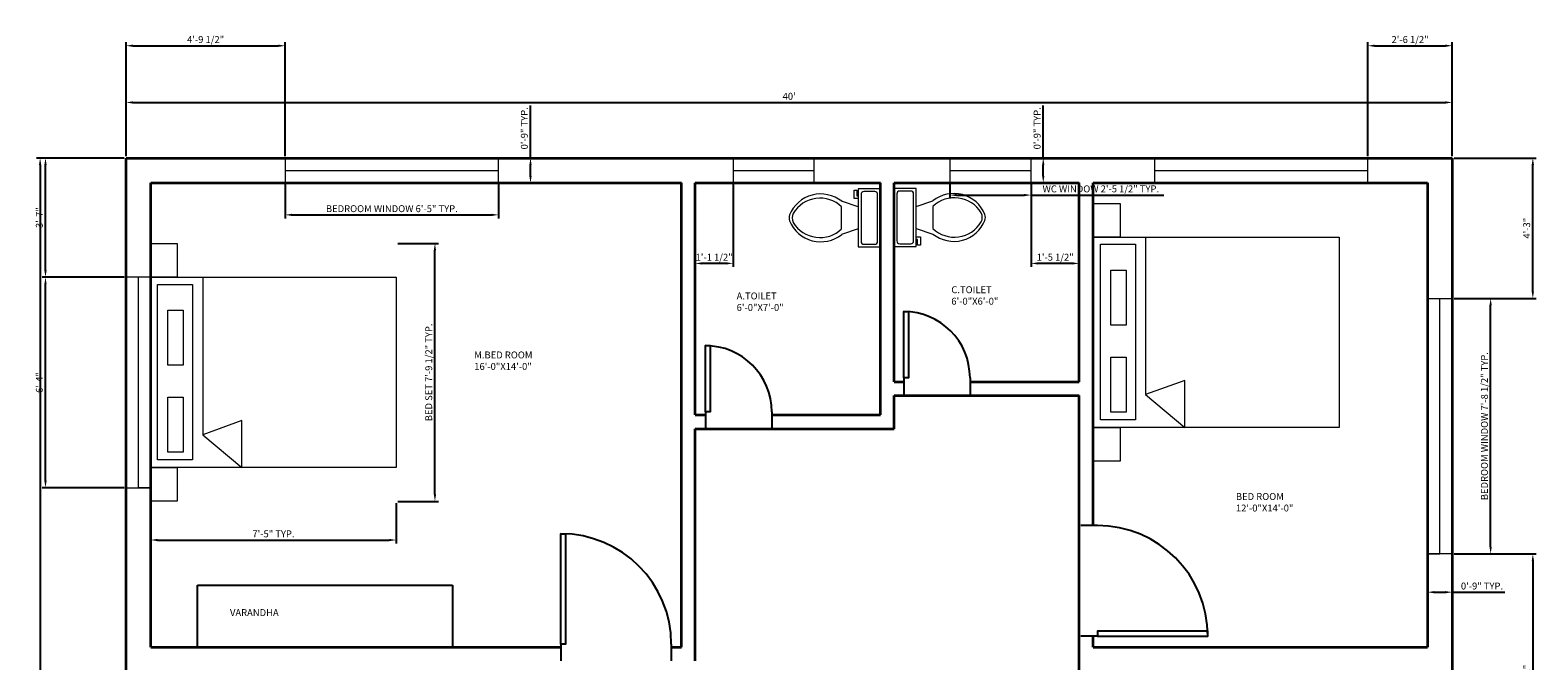
# Model space of a CAD drawing. Units: inches. Extents: x 2981 to 3526, y 1512 to 2158.
# Tile 4 of 4: x 2981 to 3526, y 1930 to 2158. Entities that reach past the tile are written whole.
import ezdxf

# ---------------------------------------------------------------- set-up
doc = ezdxf.new("R2010")
doc.units = ezdxf.units.IN
for name, color, linetype, lineweight in [('A-ANNO-DIMS', 2, 'Continuous', 18), ('A-AREA-IDEN', 7, 'Continuous', 18), ('A-DOOR', 4, 'Continuous', 25), ('A-FLOR', 7, 'Continuous', 25), ('A-FLOR-FIXT', 9, 'Continuous', 18), ('A-FURN', 8, 'Continuous', 18), ('A-GLAZ', 4, 'Continuous', 18), ('A-WALL', 7, 'Continuous', 35)]:
    doc.layers.add(name, color=color, linetype=linetype, lineweight=lineweight)
doc.styles.get("Standard").update_dxf_attribs({"font": 'arial.ttf'})
doc.dimstyles.new('ISO-25', dxfattribs={"dimtxt": 2.5, "dimasz": 2.5, "dimexe": 1.25, "dimexo": 0.625, "dimtad": 1, "dimlunit": 3, "dimtxsty": 'Standard', "dimcen": 2.5, "dimadec": 0, "dimazin": 0, "dimtfac": 1, "dimtmove": 0, "dimatfit": 3, "dimfxl": 1, "dimarcsym": 0})

# ---------------------------------------------------------------- blocks, each defined once
blk = doc.blocks.new('*U2')
for p, q in [((0, 0), (0, -6)), ((40, 0), (40, -6))]:
    blk.add_line(p, q)
blk.add_lwpolyline([(0, 0), (0, 40), (1.75, 40), (1.75, 0)], close=True)
blk.add_arc((0, 0), 40, 0, 90)
blk = doc.blocks.new('*U3')
for p, q in [((0, 0), (0, -6)), ((-40, 0), (-40, -6))]:
    blk.add_line(p, q)
blk.add_lwpolyline([(0, 0), (0, 40), (-1.75, 40), (-1.75, 0)], close=True)
blk.add_arc((0, 0), 40, 90, 180)
blk = doc.blocks.new('*U5')
for p, q in [((0, 0), (0, -6)), ((24, 0), (24, -6))]:
    blk.add_line(p, q)
blk.add_lwpolyline([(0, 0), (0, 24), (1.75, 24), (1.75, 0)], close=True)
blk.add_arc((0, 0), 24, 0, 90)
blk = doc.blocks.new('*U9')
for p, q in [((9.5, -6), (9.5, -2)), ((-10, -8.5), (-8, -8.5)), ((-10, -9.5), (-10, -8.5)), ((-7, -9.5), (-10, -9.5)), ((-8, -8.5), (-8, -8)), ((-7, -8), (-7, -9.5)), ((-4, -8), (-6, -14)), ((4, -8), (6, -14)), ((4, -14), (-4, -14))]:
    blk.add_line(p, q)
blk.add_lwpolyline([(10.5, -8), (10.5, 0), (-10.5, 0), (-10.5, -8)], close=True)
for points in [[(-9.5, -2), (-9.5, -6)], [(8.5, -1), (-8.5, -1)], [(-8.5, -7), (8.5, -7)]]:
    blk.add_lwpolyline(points)
for centre, radius, start, end in [((-8.62, -1.88), 0.884, 81.8699, 188.1301), ((8.62, -1.88), 0.884, 351.8699, 98.1301), ((-8.62, -6.12), 0.884, 171.8699, 278.1301), ((8.62, -6.12), 0.884, 261.8699, 8.1301), ((3.52, -21.58), 12.17, 141.4691, 247.9714), ((4.2, -21.82), 11.33, 136.3677, 238.9468), ((-3.52, -21.58), 12.17, 292.0284, 38.5307), ((-4.2, -21.82), 11.33, 301.053, 43.6321), ((0, -27.88), 4, 245.7318, 294.2682), ((0, -29), 4, 254.8605, 285.1395)]:
    blk.add_arc(centre, radius, start, end)
blk = doc.blocks.new('*D14')
at = {"layer": 'A-ANNO-DIMS', "color": 0, "lineweight": -2, "transparency": 16777216}
for p, q in [((3015.4, 2112.83), (3015.4, 2133.57)), ((3495.4, 2112.83), (3495.4, 2133.57)), ((3017.9, 2132.32), (3492.9, 2132.32))]:
    blk.add_line(p, q, dxfattribs=at)
at = {"layer": 'A-ANNO-DIMS', "color": 0, "transparency": 16777216}
for points in [[(3017.9, 2132.73), (3017.9, 2131.9), (3015.4, 2132.32)], [(3492.9, 2132.73), (3492.9, 2131.9), (3495.4, 2132.32)]]:
    blk.add_solid(points, dxfattribs=at)
at = {"layer": 'Defpoints', "color": 0, "transparency": 16777216}
for p in [(3495.4, 2132.32), (3015.4, 2112.2), (3495.4, 2112.2)]:
    blk.add_point(p, dxfattribs=at)
at = {"layer": 'A-ANNO-DIMS', "color": 0, "transparency": 16777216, "insert": (3255.4, 2134.22), "char_height": 2.5, "attachment_point": 5}
blk.add_mtext("40'", dxfattribs=at)
blk = doc.blocks.new('*D15')
at = {"layer": 'A-ANNO-DIMS', "color": 0, "lineweight": -2, "transparency": 16777216}
for p, q in [((3014.77, 2112.2), (2983.05, 2112.2)), ((2984.3, 2109.7), (2984.3, 1574.7)), ((3014.77, 1572.2), (2983.05, 1572.2))]:
    blk.add_line(p, q, dxfattribs=at)
at = {"layer": 'A-ANNO-DIMS', "color": 0, "transparency": 16777216}
for points in [[(2983.89, 2109.7), (2984.72, 2109.7), (2984.3, 2112.2)], [(2983.89, 1574.7), (2984.72, 1574.7), (2984.3, 1572.2)]]:
    blk.add_solid(points, dxfattribs=at)
at = {"layer": 'Defpoints', "color": 0, "transparency": 16777216}
for p in [(3015.4, 2112.2), (2984.3, 1572.2), (3015.4, 1572.2)]:
    blk.add_point(p, dxfattribs=at)
at = {"layer": 'A-ANNO-DIMS', "color": 0, "transparency": 16777216, "insert": (2982.41, 1842.2), "char_height": 2.5, "attachment_point": 5, "rotation": 90}
blk.add_mtext("45'", dxfattribs=at)
blk = doc.blocks.new('WIN-77IN-BEDROOM')
for p, q in [((0, 9), (0, 0)), ((77.2, 9), (0, 9)), ((0, 9), (0, 4.5)), ((77.2, 0), (77.2, 9)), ((0, 4.5), (77.2, 4.5)), ((0, 0), (77.2, 0))]:
    blk.add_line(p, q)
blk = doc.blocks.new('WIN-29IN-TOILET')
for p, q in [((0, 9), (0, 0)), ((29.42, 9), (0, 9)), ((0, 9), (0, 4.5)), ((29.42, 0), (29.42, 9)), ((0, 4.5), (29.42, 4.5)), ((0, 0), (29.42, 0))]:
    blk.add_line(p, q)
blk = doc.blocks.new('WIN-92IN-BEDROOM')
for p, q in [((0, 92.47), (9, 92.47)), ((0, 92.47), (0, 0)), ((4.5, 0), (4.5, 92.47)), ((9, 92.47), (9, 0)), ((9, 0), (0, 0)), ((0, 0), (4.5, 0))]:
    blk.add_line(p, q)
blk = doc.blocks.new('BED-DOUBLE-WITH-NIGHTSTANDS')
for p, q in [((18.84, 81.09), (18.84, 24.12)), ((33.02, 29.21), (18.84, 24.12)), ((33.02, 12.24), (33.02, 29.21)), ((18.84, 24.12), (33.02, 12.24))]:
    blk.add_line(p, q)
for points in [[(9.63, 93.35), (9.63, 81.1), (0.08, 81.1), (0.08, 93.35)], [(0.08, 12.24), (0.08, 81.09), (88.86, 81.09), (88.86, 12.24)], [(2.5, 15.01), (2.5, 78.54), (15.13, 78.54), (15.13, 15.01)], [(6.2, 49.25), (6.2, 69.14), (11.74, 69.14), (11.74, 49.25)], [(6.2, 17.79), (6.2, 37.68), (11.74, 37.68), (11.74, 17.79)], [(9.63, 12.24), (9.63, 0), (0, 0), (0, 12.24)]]:
    blk.add_lwpolyline(points, close=True)
blk = doc.blocks.new('*D21')
at = {"layer": 'A-ANNO-DIMS', "color": 0, "lineweight": -2, "transparency": 16777216}
for p, q in [((3113.82, 2081.29), (3128.45, 2081.29)), ((3127.2, 1990.44), (3127.2, 2078.79)), ((3113.82, 1987.94), (3128.45, 1987.94))]:
    blk.add_line(p, q, dxfattribs=at)
at = {"layer": 'A-ANNO-DIMS', "color": 0, "transparency": 16777216}
for points in [[(3126.78, 2078.79), (3127.61, 2078.79), (3127.2, 2081.29)], [(3126.78, 1990.44), (3127.61, 1990.44), (3127.2, 1987.94)]]:
    blk.add_solid(points, dxfattribs=at)
at = {"layer": 'Defpoints', "color": 0, "transparency": 16777216}
for p in [(3113.19, 2081.29), (3127.2, 2081.29), (3113.19, 1987.94)]:
    blk.add_point(p, dxfattribs=at)
at = {"layer": 'A-ANNO-DIMS', "color": 0, "transparency": 16777216, "insert": (3125.28, 2034.62), "char_height": 2.5, "attachment_point": 5, "rotation": 90}
blk.add_mtext('BED SET 7\'-9 1/2" TYP.', dxfattribs=at)
blk = doc.blocks.new('*D22')
at = {"layer": 'A-ANNO-DIMS', "color": 0, "lineweight": -2, "transparency": 16777216}
for p, q in [((3024.33, 1987.32), (3024.33, 1972.69)), ((3113.19, 1987.32), (3113.19, 1972.69)), ((3026.83, 1973.94), (3110.69, 1973.94))]:
    blk.add_line(p, q, dxfattribs=at)
at = {"layer": 'A-ANNO-DIMS', "color": 0, "transparency": 16777216}
for points in [[(3026.83, 1974.36), (3026.83, 1973.53), (3024.33, 1973.94)], [(3110.69, 1974.36), (3110.69, 1973.53), (3113.19, 1973.94)]]:
    blk.add_solid(points, dxfattribs=at)
at = {"layer": 'Defpoints', "color": 0, "transparency": 16777216}
for p in [(3024.33, 1987.94), (3113.19, 1987.94), (3113.19, 1973.94)]:
    blk.add_point(p, dxfattribs=at)
at = {"layer": 'A-ANNO-DIMS', "color": 0, "transparency": 16777216, "insert": (3068.76, 1975.84), "char_height": 2.5, "attachment_point": 5}
blk.add_mtext('7\'-5" TYP.', dxfattribs=at)
blk = doc.blocks.new('*D27')
at = {"layer": 'A-ANNO-DIMS', "color": 0, "lineweight": -2, "transparency": 16777216}
for p, q in [((3073, 2102.58), (3073, 2090.37)), ((3150.2, 2102.58), (3150.2, 2090.37)), ((3075.5, 2091.62), (3147.7, 2091.62))]:
    blk.add_line(p, q, dxfattribs=at)
at = {"layer": 'A-ANNO-DIMS', "color": 0, "transparency": 16777216}
for points in [[(3075.5, 2092.04), (3075.5, 2091.21), (3073, 2091.62)], [(3147.7, 2092.04), (3147.7, 2091.21), (3150.2, 2091.62)]]:
    blk.add_solid(points, dxfattribs=at)
at = {"layer": 'Defpoints', "color": 0, "transparency": 16777216}
for p in [(3073, 2103.2), (3150.2, 2103.2), (3150.2, 2091.62)]:
    blk.add_point(p, dxfattribs=at)
at = {"layer": 'A-ANNO-DIMS', "color": 0, "transparency": 16777216, "insert": (3111.6, 2093.54), "char_height": 2.5, "attachment_point": 5}
blk.add_mtext('BEDROOM WINDOW 6\'-5" TYP.', dxfattribs=at)
blk = doc.blocks.new('*D28')
at = {"layer": 'A-ANNO-DIMS', "color": 0, "lineweight": -2, "transparency": 16777216}
for p, q in [((3161.78, 2112.2), (3161.78, 2131.19)), ((3150.83, 2112.2), (3163.03, 2112.2)), ((3161.78, 2105.7), (3161.78, 2109.7)), ((3150.83, 2103.2), (3163.03, 2103.2))]:
    blk.add_line(p, q, dxfattribs=at)
at = {"layer": 'A-ANNO-DIMS', "color": 0, "transparency": 16777216}
for points in [[(3161.37, 2109.7), (3162.2, 2109.7), (3161.78, 2112.2)], [(3161.37, 2105.7), (3162.2, 2105.7), (3161.78, 2103.2)]]:
    blk.add_solid(points, dxfattribs=at)
at = {"layer": 'Defpoints', "color": 0, "transparency": 16777216}
for p in [(3150.2, 2112.2), (3161.78, 2112.2), (3150.2, 2103.2)]:
    blk.add_point(p, dxfattribs=at)
at = {"layer": 'A-ANNO-DIMS', "color": 0, "transparency": 16777216, "insert": (3159.88, 2122.95), "char_height": 2.5, "attachment_point": 5, "rotation": 90}
blk.add_mtext('0\'-9" TYP.', dxfattribs=at)
blk = doc.blocks.new('*D29')
at = {"layer": 'A-ANNO-DIMS', "color": 0, "lineweight": -2, "transparency": 16777216}
for p, q in [((3313.51, 2102.58), (3313.51, 2097.54)), ((3342.94, 2102.58), (3342.94, 2097.54)), ((3316.01, 2098.79), (3340.44, 2098.79)), ((3342.94, 2098.79), (3390.94, 2098.79))]:
    blk.add_line(p, q, dxfattribs=at)
at = {"layer": 'A-ANNO-DIMS', "color": 0, "transparency": 16777216}
for points in [[(3316.01, 2099.21), (3316.01, 2098.37), (3313.51, 2098.79)], [(3340.44, 2099.21), (3340.44, 2098.37), (3342.94, 2098.79)]]:
    blk.add_solid(points, dxfattribs=at)
at = {"layer": 'Defpoints', "color": 0, "transparency": 16777216}
for p in [(3313.51, 2103.2), (3342.94, 2103.2), (3342.94, 2098.79)]:
    blk.add_point(p, dxfattribs=at)
at = {"layer": 'A-ANNO-DIMS', "color": 0, "transparency": 16777216, "insert": (3368.19, 2100.71), "char_height": 2.5, "attachment_point": 5}
blk.add_mtext('WC WINDOW 2\'-5 1/2" TYP.', dxfattribs=at)
blk = doc.blocks.new('*D30')
at = {"layer": 'A-ANNO-DIMS', "color": 0, "lineweight": -2, "transparency": 16777216}
for p, q in [((3347.35, 2112.2), (3347.35, 2131.19)), ((3343.57, 2112.2), (3348.6, 2112.2)), ((3347.35, 2105.7), (3347.35, 2109.7)), ((3343.57, 2103.2), (3348.6, 2103.2))]:
    blk.add_line(p, q, dxfattribs=at)
at = {"layer": 'A-ANNO-DIMS', "color": 0, "transparency": 16777216}
for points in [[(3346.94, 2109.7), (3347.77, 2109.7), (3347.35, 2112.2)], [(3346.94, 2105.7), (3347.77, 2105.7), (3347.35, 2103.2)]]:
    blk.add_solid(points, dxfattribs=at)
at = {"layer": 'Defpoints', "color": 0, "transparency": 16777216}
for p in [(3342.94, 2112.2), (3347.35, 2112.2), (3342.94, 2103.2)]:
    blk.add_point(p, dxfattribs=at)
at = {"layer": 'A-ANNO-DIMS', "color": 0, "transparency": 16777216, "insert": (3345.45, 2122.95), "char_height": 2.5, "attachment_point": 5, "rotation": 90}
blk.add_mtext('0\'-9" TYP.', dxfattribs=at)
blk = doc.blocks.new('*D31')
at = {"layer": 'A-ANNO-DIMS', "color": 0, "lineweight": -2, "transparency": 16777216}
for p, q in [((3496.02, 2061.39), (3510.52, 2061.39)), ((3509.27, 1971.43), (3509.27, 2058.89)), ((3496.02, 1968.93), (3510.52, 1968.93))]:
    blk.add_line(p, q, dxfattribs=at)
at = {"layer": 'A-ANNO-DIMS', "color": 0, "transparency": 16777216}
for points in [[(3508.85, 2058.89), (3509.69, 2058.89), (3509.27, 2061.39)], [(3508.85, 1971.43), (3509.69, 1971.43), (3509.27, 1968.93)]]:
    blk.add_solid(points, dxfattribs=at)
at = {"layer": 'Defpoints', "color": 0, "transparency": 16777216}
for p in [(3495.4, 2061.39), (3509.27, 2061.39), (3495.4, 1968.93)]:
    blk.add_point(p, dxfattribs=at)
at = {"layer": 'A-ANNO-DIMS', "color": 0, "transparency": 16777216, "insert": (3507.35, 2015.16), "char_height": 2.5, "attachment_point": 5, "rotation": 90}
blk.add_mtext('BEDROOM WINDOW 7\'-8 1/2" TYP.', dxfattribs=at)
blk = doc.blocks.new('*D32')
at = {"layer": 'A-ANNO-DIMS', "color": 0, "lineweight": -2, "transparency": 16777216}
for p, q in [((3486.4, 1968.3), (3486.4, 1953.81)), ((3495.4, 1968.3), (3495.4, 1953.81)), ((3488.9, 1955.06), (3492.9, 1955.06)), ((3495.4, 1955.06), (3514.39, 1955.06))]:
    blk.add_line(p, q, dxfattribs=at)
at = {"layer": 'A-ANNO-DIMS', "color": 0, "transparency": 16777216}
for points in [[(3488.9, 1955.47), (3488.9, 1954.64), (3486.4, 1955.06)], [(3492.9, 1955.47), (3492.9, 1954.64), (3495.4, 1955.06)]]:
    blk.add_solid(points, dxfattribs=at)
at = {"layer": 'Defpoints', "color": 0, "transparency": 16777216}
for p in [(3486.4, 1968.93), (3495.4, 1968.93), (3495.4, 1955.06)]:
    blk.add_point(p, dxfattribs=at)
at = {"layer": 'A-ANNO-DIMS', "color": 0, "transparency": 16777216, "insert": (3506.14, 1956.96), "char_height": 2.5, "attachment_point": 5}
blk.add_mtext('0\'-9" TYP.', dxfattribs=at)
blk = doc.blocks.new('*D41')
at = {"layer": 'A-ANNO-DIMS', "color": 0, "lineweight": -2, "transparency": 16777216}
for p, q in [((3496.02, 2112.2), (3525.79, 2112.2)), ((3524.54, 2063.89), (3524.54, 2109.7)), ((3496.02, 2061.39), (3525.79, 2061.39))]:
    blk.add_line(p, q, dxfattribs=at)
at = {"layer": 'A-ANNO-DIMS', "color": 0, "transparency": 16777216}
for points in [[(3524.13, 2109.7), (3524.96, 2109.7), (3524.54, 2112.2)], [(3524.13, 2063.89), (3524.96, 2063.89), (3524.54, 2061.39)]]:
    blk.add_solid(points, dxfattribs=at)
at = {"layer": 'Defpoints', "color": 0, "transparency": 16777216}
for p in [(3495.4, 2112.2), (3524.54, 2112.2), (3495.4, 2061.39)]:
    blk.add_point(p, dxfattribs=at)
at = {"layer": 'A-ANNO-DIMS', "color": 0, "transparency": 16777216, "insert": (3522.64, 2086.8), "char_height": 2.5, "attachment_point": 5, "rotation": 90}
blk.add_mtext('4\'-3"', dxfattribs=at)
blk = doc.blocks.new('*D42')
at = {"layer": 'A-ANNO-DIMS', "color": 0, "lineweight": -2, "transparency": 16777216}
for p, q in [((3496.02, 1968.93), (3525.79, 1968.93)), ((3524.54, 1966.43), (3524.54, 1875.83)), ((3496.02, 1873.33), (3525.79, 1873.33))]:
    blk.add_line(p, q, dxfattribs=at)
at = {"layer": 'A-ANNO-DIMS', "color": 0, "transparency": 16777216}
for points in [[(3524.13, 1966.43), (3524.96, 1966.43), (3524.54, 1968.93)], [(3524.13, 1875.83), (3524.96, 1875.83), (3524.54, 1873.33)]]:
    blk.add_solid(points, dxfattribs=at)
at = {"layer": 'Defpoints', "color": 0, "transparency": 16777216}
for p in [(3495.4, 1968.93), (3495.4, 1873.33), (3524.54, 1873.33)]:
    blk.add_point(p, dxfattribs=at)
at = {"layer": 'A-ANNO-DIMS', "color": 0, "transparency": 16777216, "insert": (3522.63, 1921.13), "char_height": 2.5, "attachment_point": 5, "rotation": 90}
blk.add_mtext('7\'-11 1/2"', dxfattribs=at)
blk = doc.blocks.new('*D43')
at = {"layer": 'A-ANNO-DIMS', "color": 0, "lineweight": -2, "transparency": 16777216}
for p, q in [((3014.77, 2069.05), (2985, 2069.05)), ((2986.25, 1995.38), (2986.25, 2066.55)), ((3014.77, 1992.88), (2985, 1992.88))]:
    blk.add_line(p, q, dxfattribs=at)
at = {"layer": 'A-ANNO-DIMS', "color": 0, "transparency": 16777216}
for points in [[(2985.84, 2066.55), (2986.67, 2066.55), (2986.25, 2069.05)], [(2985.84, 1995.38), (2986.67, 1995.38), (2986.25, 1992.88)]]:
    blk.add_solid(points, dxfattribs=at)
at = {"layer": 'Defpoints', "color": 0, "transparency": 16777216}
for p in [(2986.25, 2069.05), (3015.4, 2069.05), (3015.4, 1992.88)]:
    blk.add_point(p, dxfattribs=at)
at = {"layer": 'A-ANNO-DIMS', "color": 0, "transparency": 16777216, "insert": (2984.35, 2030.96), "char_height": 2.5, "attachment_point": 5, "rotation": 90}
blk.add_mtext('6\'-4"', dxfattribs=at)
blk = doc.blocks.new('*D46')
at = {"layer": 'A-ANNO-DIMS', "color": 0, "lineweight": -2, "transparency": 16777216}
for p, q in [((3015.4, 2112.83), (3015.4, 2154.09)), ((3017.9, 2152.84), (3070.5, 2152.84)), ((3073, 2112.83), (3073, 2154.09))]:
    blk.add_line(p, q, dxfattribs=at)
at = {"layer": 'A-ANNO-DIMS', "color": 0, "transparency": 16777216}
for points in [[(3017.9, 2153.26), (3017.9, 2152.42), (3015.4, 2152.84)], [(3070.5, 2153.26), (3070.5, 2152.42), (3073, 2152.84)]]:
    blk.add_solid(points, dxfattribs=at)
at = {"layer": 'Defpoints', "color": 0, "transparency": 16777216}
for p in [(3073, 2152.84), (3015.4, 2112.2), (3073, 2112.2)]:
    blk.add_point(p, dxfattribs=at)
at = {"layer": 'A-ANNO-DIMS', "color": 0, "transparency": 16777216, "insert": (3044.2, 2154.76), "char_height": 2.5, "attachment_point": 5}
blk.add_mtext('4\'-9 1/2"', dxfattribs=at)
blk = doc.blocks.new('*D47')
at = {"layer": 'A-ANNO-DIMS', "color": 0, "lineweight": -2, "transparency": 16777216}
for p, q in [((3221.4, 2102.58), (3221.4, 2072.81)), ((3235.08, 2102.58), (3235.08, 2072.81)), ((3232.58, 2074.06), (3223.9, 2074.06))]:
    blk.add_line(p, q, dxfattribs=at)
at = {"layer": 'A-ANNO-DIMS', "color": 0, "transparency": 16777216}
for points in [[(3223.9, 2074.47), (3223.9, 2073.64), (3221.4, 2074.06)], [(3232.58, 2074.47), (3232.58, 2073.64), (3235.08, 2074.06)]]:
    blk.add_solid(points, dxfattribs=at)
at = {"layer": 'Defpoints', "color": 0, "transparency": 16777216}
for p in [(3221.4, 2103.2), (3235.08, 2103.2), (3221.4, 2074.06)]:
    blk.add_point(p, dxfattribs=at)
at = {"layer": 'A-ANNO-DIMS', "color": 0, "transparency": 16777216, "insert": (3228.24, 2075.98), "char_height": 2.5, "attachment_point": 5}
blk.add_mtext('1\'-1 1/2"', dxfattribs=at)
blk = doc.blocks.new('*D48')
at = {"layer": 'A-ANNO-DIMS', "color": 0, "lineweight": -2, "transparency": 16777216}
for p, q in [((3342.94, 2102.58), (3342.94, 2072.81)), ((3360.4, 2102.58), (3360.4, 2072.81)), ((3357.9, 2074.06), (3345.44, 2074.06))]:
    blk.add_line(p, q, dxfattribs=at)
at = {"layer": 'A-ANNO-DIMS', "color": 0, "transparency": 16777216}
for points in [[(3345.44, 2074.47), (3345.44, 2073.64), (3342.94, 2074.06)], [(3357.9, 2074.47), (3357.9, 2073.64), (3360.4, 2074.06)]]:
    blk.add_solid(points, dxfattribs=at)
at = {"layer": 'Defpoints', "color": 0, "transparency": 16777216}
for p in [(3342.94, 2103.2), (3360.4, 2103.2), (3342.94, 2074.06)]:
    blk.add_point(p, dxfattribs=at)
at = {"layer": 'A-ANNO-DIMS', "color": 0, "transparency": 16777216, "insert": (3351.67, 2075.98), "char_height": 2.5, "attachment_point": 5}
blk.add_mtext('1\'-5 1/2"', dxfattribs=at)
blk = doc.blocks.new('*D49')
at = {"layer": 'A-ANNO-DIMS', "color": 0, "lineweight": -2, "transparency": 16777216}
for p, q in [((3464.81, 2112.83), (3464.81, 2154.09)), ((3467.31, 2152.84), (3492.9, 2152.84)), ((3495.4, 2112.83), (3495.4, 2154.09))]:
    blk.add_line(p, q, dxfattribs=at)
at = {"layer": 'A-ANNO-DIMS', "color": 0, "transparency": 16777216}
for points in [[(3467.31, 2153.26), (3467.31, 2152.42), (3464.81, 2152.84)], [(3492.9, 2153.26), (3492.9, 2152.42), (3495.4, 2152.84)]]:
    blk.add_solid(points, dxfattribs=at)
at = {"layer": 'Defpoints', "color": 0, "transparency": 16777216}
for p in [(3495.4, 2152.84), (3464.81, 2112.2), (3495.4, 2112.2)]:
    blk.add_point(p, dxfattribs=at)
at = {"layer": 'A-ANNO-DIMS', "color": 0, "transparency": 16777216, "insert": (3480.11, 2154.76), "char_height": 2.5, "attachment_point": 5}
blk.add_mtext('2\'-6 1/2"', dxfattribs=at)
blk = doc.blocks.new('*D50')
at = {"layer": 'A-ANNO-DIMS', "color": 0, "lineweight": -2, "transparency": 16777216}
for p, q in [((3014.77, 2112.2), (2985, 2112.2)), ((2986.25, 2071.55), (2986.25, 2109.7)), ((3014.77, 2069.05), (2985, 2069.05))]:
    blk.add_line(p, q, dxfattribs=at)
at = {"layer": 'A-ANNO-DIMS', "color": 0, "transparency": 16777216}
for points in [[(2985.84, 2109.7), (2986.67, 2109.7), (2986.25, 2112.2)], [(2985.84, 2071.55), (2986.67, 2071.55), (2986.25, 2069.05)]]:
    blk.add_solid(points, dxfattribs=at)
at = {"layer": 'Defpoints', "color": 0, "transparency": 16777216}
for p in [(2986.25, 2112.2), (3015.4, 2112.2), (3015.4, 2069.05)]:
    blk.add_point(p, dxfattribs=at)
at = {"layer": 'A-ANNO-DIMS', "color": 0, "transparency": 16777216, "insert": (2984.35, 2090.63), "char_height": 2.5, "attachment_point": 5, "rotation": 90}
blk.add_mtext('3\'-7"', dxfattribs=at)

msp = doc.modelspace()

# ---------------------------------------------------------------- linework, layer by layer
at = {"layer": 'A-FLOR'}
for p, q in [((3041.241, 1935.202), (3041.241, 1957.601)), ((3041.241, 1957.601), (3133.515, 1957.601)), ((3133.515, 1957.601), (3133.515, 1935.202))]:
    msp.add_line(p, q, dxfattribs=at)
at = {"layer": 'A-GLAZ'}
for p, q in [((3024.411, 2069.048), (3015.399, 2069.048)), ((3015.399, 2069.048), (3015.399, 1992.878)), ((3019.865, 1992.878), (3019.905, 2069.048)), ((3015.399, 1992.878), (3024.331, 1992.878)), ((3024.331, 1992.878), (3019.865, 1992.878))]:
    msp.add_line(p, q, dxfattribs=at)
at = {"layer": 'A-WALL'}
for p, q in [((3015.399, 2112.202), (3495.399, 2112.202)), ((3015.399, 1572.202), (3015.399, 2112.202)), ((3495.399, 2112.202), (3495.399, 1572.202)), ((3024.399, 2103.202), (3216.399, 2103.202)), ((3024.399, 1935.202), (3024.399, 2103.202)), ((3216.399, 1935.202), (3216.399, 2103.202)), ((3221.399, 2019.202), (3221.399, 2103.202)), ((3221.399, 2103.202), (3288.399, 2103.202)), ((3288.399, 2019.202), (3288.399, 2103.202)), ((3293.399, 2103.202), (3360.399, 2103.202)), ((3293.399, 2031.202), (3293.399, 2103.202)), ((3360.399, 2031.202), (3360.399, 2103.202)), ((3365.399, 2103.202), (3486.399, 2103.202)), ((3365.399, 1979.181), (3365.399, 2103.202)), ((3486.399, 2103.202), (3486.399, 1935.202)), ((3293.399, 2031.202), (3296.846, 2031.202)), ((3320.846, 2031.202), (3360.399, 2031.202)), ((3365.399, 2026.202), (3365.399, 2031.202)), ((3293.399, 2019.202), (3293.399, 2026.202)), ((3293.399, 2026.202), (3360.399, 2026.202)), ((3360.399, 1745.202), (3360.399, 2026.202)), ((3221.399, 2019.202), (3225.109, 2019.202)), ((3249.109, 2019.202), (3288.399, 2019.202)), ((3293.399, 2014.202), (3293.399, 2019.202)), ((3221.399, 1930.202), (3221.399, 2014.202)), ((3221.399, 2014.202), (3288.399, 2014.202)), ((3288.399, 2014.202), (3293.399, 2014.202)), ((3365.399, 1935.202), (3365.399, 1939.181)), ((3024.399, 1935.202), (3172.743, 1935.202)), ((3024.399, 1935.202), (3172.743, 1935.202)), ((3212.743, 1935.202), (3216.399, 1935.202)), ((3212.743, 1935.202), (3216.399, 1935.202)), ((3365.399, 1935.202), (3486.399, 1935.202))]:
    msp.add_line(p, q, dxfattribs=at)

# ---------------------------------------------------------------- block references
at = {"layer": 'A-DOOR'}
for name, p in [('*U5', (3296.846, 2032.639)), ('*U5', (3225.109, 2020.286)), ('*U2', (3172.743, 1936.211))]:
    msp.add_blockref(name, p, dxfattribs=at)
at = {"layer": 'A-DOOR', "rotation": 270}
msp.add_blockref('*U3', (3366.937, 1939.181), dxfattribs=at)
at = {"layer": 'A-FLOR-FIXT'}
for p, rotation in [((3288.399, 2090.537), 270.0000000000003), ((3293.399, 2090.693), 90.00000000000036)]:
    msp.add_blockref('*U9', p, dxfattribs=dict(at, rotation=rotation))
at = {"layer": 'A-FURN'}
for p in [(3365.572, 2002.441), (3024.331, 1987.944)]:
    msp.add_blockref('BED-DOUBLE-WITH-NIGHTSTANDS', p, dxfattribs=at)
at = {"layer": 'A-GLAZ'}
for name, p in [('WIN-77IN-BEDROOM', (3073.002, 2103.202)), ('WIN-29IN-TOILET', (3235.079, 2103.202)), ('WIN-29IN-TOILET', (3313.515, 2103.202)), ('WIN-77IN-BEDROOM', (3387.613, 2103.202)), ('WIN-92IN-BEDROOM', (3486.399, 1968.927))]:
    msp.add_blockref(name, p, dxfattribs=at)

# ---------------------------------------------------------------- texts
at = {"layer": 'A-AREA-IDEN', "char_height": 2.5, "attachment_point": 1}
for s, width, insert in [('A.TOILET\\P6\'-0"X7\'-0"', 35.95085, (3236.388, 2063.529)), ('C.TOILET\\P6\'-0"X6\'-0"', 40.9686, (3314.088, 2065.782)), ('M.BED ROOM\\P16\'-0"X14\'-0"', 49.38491, (3141.428, 2042.178)), ('BED ROOM\\P12\'-0"X14\'-0"', 47.16292, (3417.08, 1990.935)), ('VARANDHA', 41.80757, (3053.022, 1948.916))]:
    msp.add_mtext_dynamic_manual_height_columns(s, width=width, gutter_width=12.5, heights=[0], dxfattribs=dict(at, insert=insert))

# ---------------------------------------------------------------- dimensions: what is measured, and where the dimension line sits
at = {"layer": 'A-ANNO-DIMS'}
for base, p1, p2, override, picture, middle in [((3073.002, 2152.838), (3015.399, 2112.202), (3073.002, 2112.202), {"dimdec": 1, "dimlfac": 1, "dimrnd": 0, "dimzin": 1, "dimdsep": 46, "dimlunit": 4, "dimfrac": 2}, '*D46', (3044.201, 2154.756)), ((3495.399, 2152.838), (3464.814, 2112.202), (3495.399, 2112.202), {"dimdec": 1, "dimlfac": 1, "dimrnd": 0, "dimzin": 1, "dimdsep": 46, "dimlunit": 4, "dimfrac": 2}, '*D49', (3480.106, 2154.756)), ((3495.399, 2132.315), (3015.399, 2112.202), (3495.399, 2112.202), {"dimclrd": 0, "dimclre": 0, "dimclrt": 0}, '*D14', (3255.399, 2134.217))]:
    dim = msp.add_linear_dim(base=base, p1=p1, p2=p2, dimstyle='ISO-25', override=override, dxfattribs=at)
    dim.commit()
    dim.dimension.update_dxf_attribs({"geometry": picture, "text_midpoint": middle})
for base, p1, p2, text, picture, middle in [((3161.783, 2112.202), (3150.203, 2103.202), (3150.203, 2112.202), '<> TYP.', '*D28', (3159.881, 2122.947)), ((3347.354, 2112.202), (3342.94, 2103.202), (3342.94, 2112.202), '<> TYP.', '*D30', (3345.452, 2122.947)), ((3127.195, 2081.289), (3113.194, 1987.944), (3113.194, 2081.289), 'BED SET <> TYP.', '*D21', (3125.278, 2034.617)), ((3509.27, 2061.395), (3495.399, 1968.927), (3495.399, 2061.395), 'BEDROOM WINDOW <> TYP.', '*D31', (3507.351, 2015.161))]:
    dim = msp.add_linear_dim(base=base, p1=p1, p2=p2, angle=90, text=text, dimstyle='ISO-25', override={"dimdec": 1, "dimlfac": 1, "dimrnd": 0, "dimzin": 1, "dimdsep": 46, "dimlunit": 4, "dimfrac": 2}, dxfattribs=at)
    dim.commit()
    dim.dimension.update_dxf_attribs({"geometry": picture, "text_midpoint": middle})
for base, p1, p2, angle, override, picture, middle in [((2984.303, 1572.202), (3015.399, 2112.202), (3015.399, 1572.202), 90, {"dimclrd": 0, "dimclre": 0, "dimclrt": 0}, '*D15', (2982.407, 1842.202)), ((2986.254, 2112.202), (3015.399, 2069.048), (3015.399, 2112.202), 90, {"dimdec": 1, "dimlfac": 1, "dimrnd": 0, "dimzin": 1, "dimdsep": 46, "dimlunit": 4, "dimfrac": 2}, '*D50', (2984.352, 2090.625)), ((3524.544, 2112.202), (3495.399, 2061.395), (3495.399, 2112.202), 90, {"dimdec": 1, "dimlfac": 1, "dimrnd": 0, "dimzin": 1, "dimdsep": 46, "dimlunit": 4, "dimfrac": 2}, '*D41', (3522.642, 2086.799)), ((3221.399, 2074.057), (3235.079, 2103.202), (3221.399, 2103.202), 180, {"dimdec": 1, "dimlfac": 1, "dimrnd": 0, "dimzin": 1, "dimdsep": 46, "dimlunit": 4, "dimfrac": 2}, '*D47', (3228.239, 2075.975)), ((3342.94, 2074.057), (3360.399, 2103.202), (3342.94, 2103.202), 180, {"dimdec": 1, "dimlfac": 1, "dimrnd": 0, "dimzin": 1, "dimdsep": 46, "dimlunit": 4, "dimfrac": 2}, '*D48', (3351.67, 2075.975)), ((2986.254, 2069.048), (3015.399, 1992.878), (3015.399, 2069.048), 90, {"dimdec": 1, "dimlfac": 1, "dimrnd": 0, "dimzin": 1, "dimdsep": 46, "dimlunit": 4, "dimfrac": 2}, '*D43', (2984.353, 2030.963)), ((3524.544, 1873.333), (3495.399, 1968.927), (3495.399, 1873.333), 90, {"dimdec": 1, "dimlfac": 1, "dimrnd": 0, "dimzin": 1, "dimdsep": 46, "dimlunit": 4, "dimfrac": 2}, '*D42', (3522.627, 1921.13))]:
    dim = msp.add_linear_dim(base=base, p1=p1, p2=p2, angle=angle, dimstyle='ISO-25', override=override, dxfattribs=at)
    dim.commit()
    dim.dimension.update_dxf_attribs({"geometry": picture, "text_midpoint": middle})
for base, p1, p2, text, picture, middle in [((3342.94, 2098.789), (3313.515, 2103.202), (3342.94, 2103.202), 'WC WINDOW <> TYP.', '*D29', (3368.19, 2100.707)), ((3150.203, 2091.622), (3073.002, 2103.202), (3150.203, 2103.202), 'BEDROOM WINDOW <> TYP.', '*D27', (3111.602, 2093.541)), ((3113.194, 1973.943), (3024.331, 1987.944), (3113.194, 1987.944), '<> TYP.', '*D22', (3068.762, 1975.839)), ((3495.399, 1955.057), (3486.399, 1968.927), (3495.399, 1968.927), '<> TYP.', '*D32', (3506.144, 1956.958))]:
    dim = msp.add_linear_dim(base=base, p1=p1, p2=p2, text=text, dimstyle='ISO-25', override={"dimdec": 1, "dimlfac": 1, "dimrnd": 0, "dimzin": 1, "dimdsep": 46, "dimlunit": 4, "dimfrac": 2}, dxfattribs=at)
    dim.commit()
    dim.dimension.update_dxf_attribs({"geometry": picture, "text_midpoint": middle})

doc.saveas('drawing.dxf')
